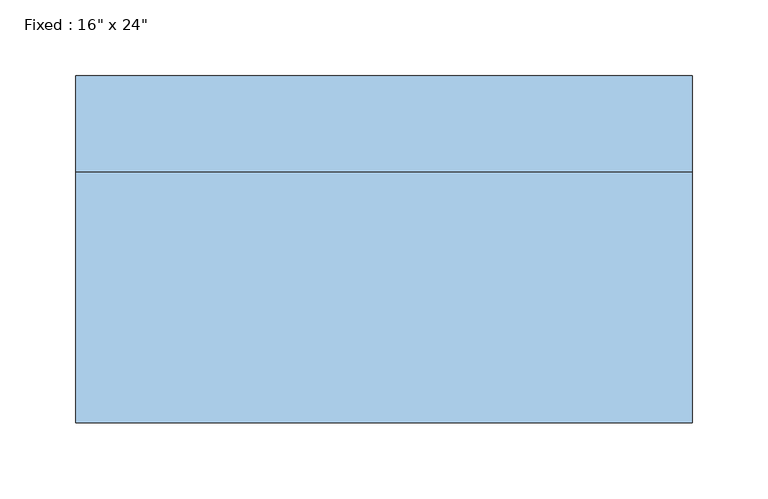
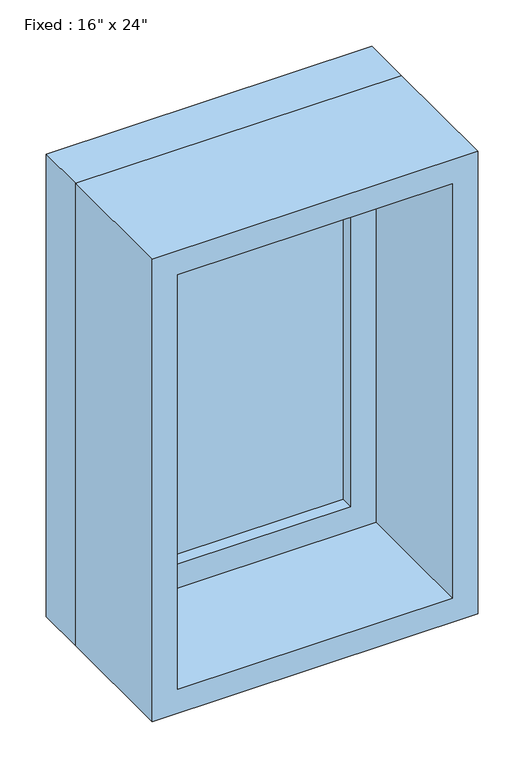
"""IFC4 building model written with IfcOpenShell, lengths in millimetres: window geometry."""

from ifc_helpers import new_model, si_unit, frame, origin, place, context, project, spatial, polyline, outline, extrude, source, transform, mapped, element, save


def window_aa618e30(model_context):
    return source(origin(), model_context, "Body", "SweptSolid", [
        extrude(outline(polyline([(101.6, 66.675), (-177.8, 66.675), (-177.8, 79.375), (101.6, 79.375), (101.6, 66.675)])), frame((0.0, 0.0, 977.9), z_axis=(0.0, 0.0, 1.0), x_axis=(1.0, 0.0, 0.0)), (0.0, 0.0, 1.0), 482.6),
        extrude(outline(polyline([(1504.95, -222.25), (933.45, -222.25), (933.45, 146.05), (1504.95, 146.05), (1504.95, -222.25)]), holes=[polyline([(1460.5, -177.8), (1460.5, 101.6), (977.9, 101.6), (977.9, -177.8), (1460.5, -177.8)])]), frame((0.0, 50.8, 0.0), z_axis=(0.0, 1.0, 0.0), x_axis=(0.0, 0.0, 1.0)), (0.0, 0.0, 1.0), 44.45),
        extrude(outline(polyline([(1524.0, -241.3), (914.4, -241.3), (914.4, 165.1), (1524.0, 165.1), (1524.0, -241.3)]), holes=[polyline([(1492.25, -209.55), (1492.25, 133.35), (946.15, 133.35), (946.15, -209.55), (1492.25, -209.55)])]), frame((0.0, -114.3, 0.0), z_axis=(0.0, 1.0, 0.0), x_axis=(0.0, 0.0, 1.0)), (0.0, 0.0, 1.0), 165.1),
        extrude(outline(polyline([(1524.0, 165.1), (1524.0, -241.3), (914.4, -241.3), (914.4, 165.1), (1524.0, 165.1)]), holes=[polyline([(1504.95, 146.05), (933.45, 146.05), (933.45, -222.25), (1504.95, -222.25), (1504.95, 146.05)])]), frame((0.0, 50.8, 0.0), z_axis=(0.0, 1.0, 0.0), x_axis=(0.0, 0.0, 1.0)), (0.0, 0.0, 1.0), 63.5),
    ])


if __name__ == "__main__":
    model = new_model("IFC4")
    model_context = context("Model", 3, world=origin())
    ifc_project = project(units=[si_unit("LENGTHUNIT", "METRE", prefix="MILLI")], contexts=[model_context])
    site = spatial("IfcSite", under=ifc_project)
    building = spatial("IfcBuilding", under=site)
    placement = place(None, origin())
    window_shape = window_aa618e30(model_context)
    element("IfcWindow", 1, ObjectType="Fixed : 16\" x 24\"", at=placement, inside=building, context=model_context, shape_type="MappedRepresentation", body=[
        mapped(window_shape, transform((0.0, 0.0, 0.0), x_axis=(1.0, 0.0, 0.0), y_axis=(0.0, 1.0, 0.0), z_axis=(0.0, 0.0, 1.0))),
    ])
    save(model, "model.ifc")

# Revit data of these elements
# Type "Fixed : 16\" x 24\""
#   Type Mark = "4"
#   Construction Type Id = "GSP4R"
#   Assembly Code = "B2020100"
#   Analytic Construction = "1/8 in Pilkington single glazing"
#   Visual Light Transmittance = 0.9
#   Solar Heat Gain Coefficient = 0.78
#   Heat Transfer Coefficient (U) = 0.6496 BTU/(h·ft²·°F)
#   Height = 2' - 0"
#   Default Sill Height = 3' - 0"
#   Width = 1' - 4"
#   Window Inset = 0' - 0 3/4"
#   Define Thermal Properties by = 1
#   Define Thermal Properties by = 1
#   Glass Pane Material = Glass
#   Sash Material = Sash
#   Wall Closure = (empty or 0)
# Element 1 (IfcWindow, "Fixed : 16\" x 24\"")
#   Materials on its faces: "Sash", "Glass"
# Materials
#   "Glass": class "Glass", colour RGB 0 128 192, transparency 0.75, Description = "Soda Lime Glass", Cost = 0
#   "Sash": class "Wood", colour RGB 224 178 126, transparency 0, Cost = 0
